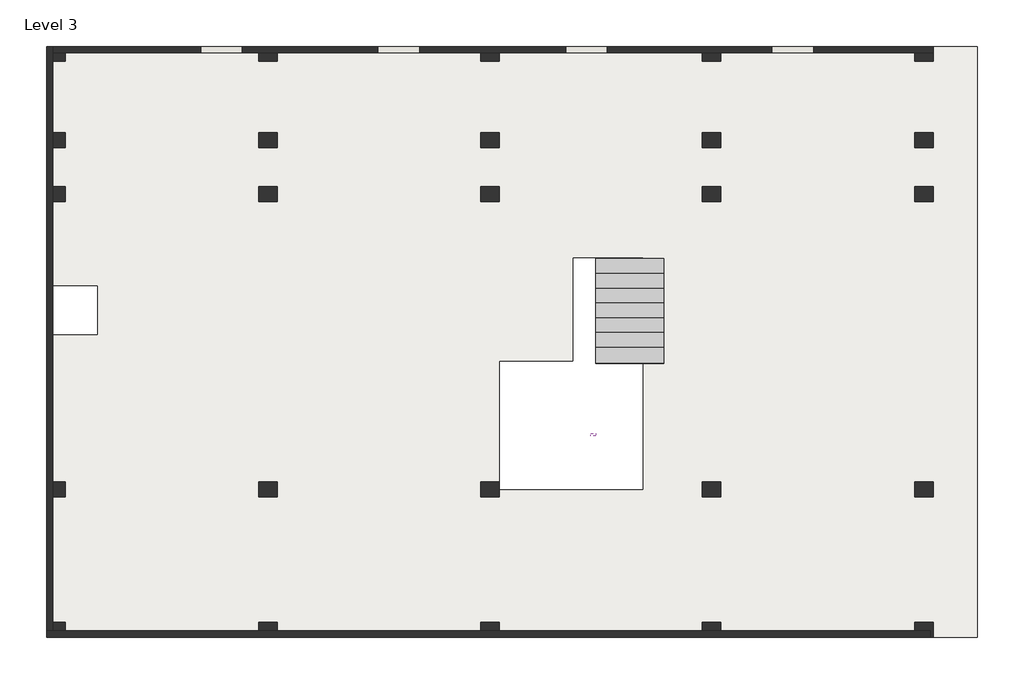
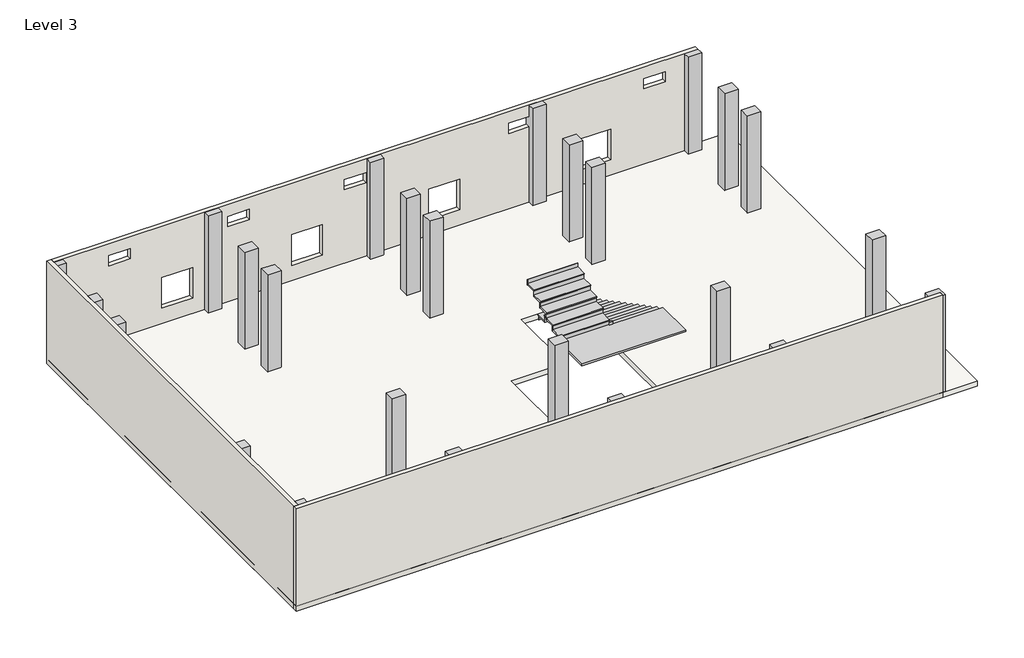
# One storey: 25 columns, 3 walls, 1 member, 1 slab, 1 stair flight.
"""IFC4 building model written with IfcOpenShell, lengths in millimetres."""

from ifc_helpers import new_model, si_unit, frame, origin, place, context, project, spatial, polyline, outline, extrude, faceted_brep, transform, mapped, element, save
from components import column_family_column_family_39b5c8c6, stair_flight_2e5e19c8

model = new_model("IFC4")

# Units and contexts
model_context = context("Model", 3, world=origin())
ifc_project = project(units=[si_unit("LENGTHUNIT", "METRE", prefix="MILLI")], contexts=[model_context])

# Site, building, storey
site = spatial("IfcSite", under=ifc_project)
building = spatial("IfcBuilding", under=site)
storey = spatial("IfcBuildingStorey", under=building, Name="Level 3", Elevation=6096.0)

# Columns
placement = place(None, origin())
element("IfcColumn", 1, ObjectType="column family : column family", at=placement, inside=storey, context=model_context, shape_type="SweptSolid", body=[
    extrude(outline(polyline([(-12064.0425534, 2926.4168492), (-12318.0425534, 2926.4168492), (-12318.0425534, 3104.2168492), (-12064.0425534, 3104.2168492), (-12064.0425534, 2926.4168492)])), frame((0.0, 0.0, 6101.0), z_axis=(0.0, 0.0, 1.0), x_axis=(1.0, 0.0, 0.0)), (0.0, 0.0, 1.0), 3038.0),
])
element("IfcColumn", 2, ObjectType="column family : column family", at=placement, inside=storey, context=model_context, shape_type="SweptSolid", body=[
    extrude(outline(polyline([(-7682.5425534, 2926.4168492), (-8063.5425534, 2926.4168492), (-8063.5425534, 3104.2168492), (-7682.5425534, 3104.2168492), (-7682.5425534, 2926.4168492)])), frame((0.0, 0.0, 6101.0), z_axis=(0.0, 0.0, 1.0), x_axis=(1.0, 0.0, 0.0)), (0.0, 0.0, 1.0), 3038.0),
])
element("IfcColumn", 3, ObjectType="column family : column family", at=placement, inside=storey, context=model_context, shape_type="SweptSolid", body=[
    extrude(outline(polyline([(-3110.5425534, 2926.4168492), (-3491.5425534, 2926.4168492), (-3491.5425534, 3104.2168492), (-3110.5425534, 3104.2168492), (-3110.5425534, 2926.4168492)])), frame((0.0, 0.0, 6101.0), z_axis=(0.0, 0.0, 1.0), x_axis=(1.0, 0.0, 0.0)), (0.0, 0.0, 1.0), 3038.0),
])
element("IfcColumn", 4, ObjectType="column family : column family", at=placement, inside=storey, context=model_context, shape_type="Brep", body=[
    faceted_brep([(1461.4574466, 2926.4168492, 6101.0), (1080.4574466, 2926.4168492, 6101.0), (1080.4574466, 3104.2168492, 6101.0), (1461.4574466, 3104.2168492, 6101.0), (1461.4574466, 2926.4168492, 9139.0), (1461.4574466, 3104.2168492, 9139.0), (1080.4574466, 2926.4168492, 9139.0), (1080.4574466, 3104.2168492, 9139.0), (1080.4574466, 3104.2168492, 8797.4055795), (1080.4574466, 3231.2168492, 8797.4055795), (1080.4574466, 3231.2168492, 8492.6055795), (1080.4574466, 3104.2168492, 8492.6055795), (1118.5574466, 3231.2168492, 8797.4055795), (1118.5574466, 3231.2168492, 8492.6055795), (1118.5574466, 3104.2168492, 8492.6055795), (1118.5574466, 3104.2168492, 8797.4055795)], [[[0, 1, 2, 3]], [[4, 0, 3, 5]], [[1, 0, 4, 6]], [[1, 6, 7, 8, 9, 10, 11, 2]], [[10, 9, 12, 13]], [[6, 4, 5, 7]], [[14, 15, 8, 7, 5, 3, 2, 11]], [[13, 14, 11, 10]], [[15, 14, 13, 12]], [[15, 12, 9, 8]]]),
])
element("IfcColumn", 5, ObjectType="column family : column family", at=placement, inside=storey, context=model_context, shape_type="SweptSolid", body=[
    extrude(outline(polyline([(5842.9574466, 2926.4168492), (5461.9574466, 2926.4168492), (5461.9574466, 3104.2168492), (5842.9574466, 3104.2168492), (5842.9574466, 2926.4168492)])), frame((0.0, 0.0, 6101.0), z_axis=(0.0, 0.0, 1.0), x_axis=(1.0, 0.0, 0.0)), (0.0, 0.0, 1.0), 3038.0),
])
element("IfcColumn", 6, ObjectType="column family : column family", at=placement, inside=storey, context=model_context, shape_type="SweptSolid", body=[
    extrude(outline(polyline([(-12064.0425534, 335.6168492), (-12064.0425534, 30.8168492), (-12318.0425534, 30.8168492), (-12318.0425534, 335.6168492), (-12064.0425534, 335.6168492)])), frame((0.0, 0.0, 6101.0), z_axis=(0.0, 0.0, 1.0), x_axis=(1.0, 0.0, 0.0)), (0.0, 0.0, 1.0), 3038.0),
])
element("IfcColumn", 7, ObjectType="column family : column family", at=placement, inside=storey, context=model_context, shape_type="SweptSolid", body=[
    extrude(outline(polyline([(-12064.0425534, 1449.6754758), (-12064.0425534, 1144.8754758), (-12318.0425534, 1144.8754758), (-12318.0425534, 1449.6754758), (-12064.0425534, 1449.6754758)])), frame((0.0, 0.0, 6101.0), z_axis=(0.0, 0.0, 1.0), x_axis=(1.0, 0.0, 0.0)), (0.0, 0.0, 1.0), 3038.0),
])
element("IfcColumn", 8, ObjectType="column family : column family", at=placement, inside=storey, context=model_context, shape_type="SweptSolid", body=[
    extrude(outline(polyline([(-12064.0425534, -5760.3831508), (-12064.0425534, -6065.1831508), (-12318.0425534, -6065.1831508), (-12318.0425534, -5760.3831508), (-12064.0425534, -5760.3831508)])), frame((0.0, 0.0, 6101.0), z_axis=(0.0, 0.0, 1.0), x_axis=(1.0, 0.0, 0.0)), (0.0, 0.0, 1.0), 3038.0),
])
element("IfcColumn", 9, ObjectType="column family : column family", at=placement, inside=storey, context=model_context, shape_type="SweptSolid", body=[
    extrude(outline(polyline([(-12064.0425534, -8655.9831508), (-12064.0425534, -8833.7831508), (-12318.0425534, -8833.7831508), (-12318.0425534, -8655.9831508), (-12064.0425534, -8655.9831508)])), frame((0.0, 0.0, 6101.0), z_axis=(0.0, 0.0, 1.0), x_axis=(1.0, 0.0, 0.0)), (0.0, 0.0, 1.0), 3038.0),
])
element("IfcColumn", 10, ObjectType="column family : column family", at=placement, inside=storey, context=model_context, shape_type="SweptSolid", body=[
    extrude(outline(polyline([(5842.9574466, 335.6168492), (5842.9574466, 30.8168492), (5461.9574466, 30.8168492), (5461.9574466, 335.6168492), (5842.9574466, 335.6168492)])), frame((0.0, 0.0, 6101.0), z_axis=(0.0, 0.0, 1.0), x_axis=(1.0, 0.0, 0.0)), (0.0, 0.0, 1.0), 3038.0),
])
element("IfcColumn", 11, ObjectType="column family : column family", at=placement, inside=storey, context=model_context, shape_type="SweptSolid", body=[
    extrude(outline(polyline([(5842.9574466, 1449.6754758), (5842.9574466, 1144.8754758), (5461.9574466, 1144.8754758), (5461.9574466, 1449.6754758), (5842.9574466, 1449.6754758)])), frame((0.0, 0.0, 6101.0), z_axis=(0.0, 0.0, 1.0), x_axis=(1.0, 0.0, 0.0)), (0.0, 0.0, 1.0), 3038.0),
])
element("IfcColumn", 12, ObjectType="column family : column family", at=placement, inside=storey, context=model_context, shape_type="SweptSolid", body=[
    extrude(outline(polyline([(5842.9574466, -5760.3831508), (5842.9574466, -6065.1831508), (5461.9574466, -6065.1831508), (5461.9574466, -5760.3831508), (5842.9574466, -5760.3831508)])), frame((0.0, 0.0, 6101.0), z_axis=(0.0, 0.0, 1.0), x_axis=(1.0, 0.0, 0.0)), (0.0, 0.0, 1.0), 3038.0),
])
element("IfcColumn", 13, ObjectType="column family : column family", at=placement, inside=storey, context=model_context, shape_type="SweptSolid", body=[
    extrude(outline(polyline([(5842.9574466, -8655.9831508), (5842.9574466, -8960.7831508), (5779.4574466, -8960.7831508), (5779.4574466, -8833.7831508), (5461.9574466, -8833.7831508), (5461.9574466, -8655.9831508), (5842.9574466, -8655.9831508)])), frame((0.0, 0.0, 6101.0), z_axis=(0.0, 0.0, 1.0), x_axis=(1.0, 0.0, 0.0)), (0.0, 0.0, 1.0), 3038.0),
])
element("IfcColumn", 14, ObjectType="column family : column family", at=placement, inside=storey, context=model_context, shape_type="SweptSolid", body=[
    extrude(outline(polyline([(-8063.5425534, -8655.9831508), (-7682.5425534, -8655.9831508), (-7682.5425534, -8833.7831508), (-8063.5425534, -8833.7831508), (-8063.5425534, -8655.9831508)])), frame((0.0, 0.0, 6101.0), z_axis=(0.0, 0.0, 1.0), x_axis=(1.0, 0.0, 0.0)), (0.0, 0.0, 1.0), 3038.0),
])
element("IfcColumn", 15, ObjectType="column family : column family", at=placement, inside=storey, context=model_context, shape_type="SweptSolid", body=[
    extrude(outline(polyline([(-3491.5425534, -8655.9831508), (-3110.5425534, -8655.9831508), (-3110.5425534, -8833.7831508), (-3491.5425534, -8833.7831508), (-3491.5425534, -8655.9831508)])), frame((0.0, 0.0, 6101.0), z_axis=(0.0, 0.0, 1.0), x_axis=(1.0, 0.0, 0.0)), (0.0, 0.0, 1.0), 3038.0),
])
element("IfcColumn", 16, ObjectType="column family : column family", at=placement, inside=storey, context=model_context, shape_type="SweptSolid", body=[
    extrude(outline(polyline([(1080.4574466, -8655.9831508), (1461.4574466, -8655.9831508), (1461.4574466, -8833.7831508), (1080.4574466, -8833.7831508), (1080.4574466, -8655.9831508)])), frame((0.0, 0.0, 6101.0), z_axis=(0.0, 0.0, 1.0), x_axis=(1.0, 0.0, 0.0)), (0.0, 0.0, 1.0), 3038.0),
])
column_family_column_family_shape = column_family_column_family_39b5c8c6(model_context)
element("IfcColumn", 17, ObjectType="column family : column family", at=placement, inside=storey, context=model_context, shape_type="MappedRepresentation", body=[
    mapped(column_family_column_family_shape, transform((-7928.6704001, 183.2168492, 0.0), x_axis=(1.0, 0.0, 0.0), y_axis=(0.0, 1.0, 0.0), z_axis=(0.0, 0.0, 1.0))),
])
element("IfcColumn", 18, ObjectType="column family : column family", at=placement, inside=storey, context=model_context, shape_type="MappedRepresentation", body=[
    mapped(column_family_column_family_shape, transform((-3356.6704001, 183.2168492, 0.0), x_axis=(1.0, 0.0, 0.0), y_axis=(0.0, 1.0, 0.0), z_axis=(0.0, 0.0, 1.0))),
])
element("IfcColumn", 19, ObjectType="column family : column family", at=placement, inside=storey, context=model_context, shape_type="MappedRepresentation", body=[
    mapped(column_family_column_family_shape, transform((1215.3295999, 183.2168492, 0.0), x_axis=(1.0, 0.0, 0.0), y_axis=(0.0, 1.0, 0.0), z_axis=(0.0, 0.0, 1.0))),
])
element("IfcColumn", 20, ObjectType="column family : column family", at=placement, inside=storey, context=model_context, shape_type="MappedRepresentation", body=[
    mapped(column_family_column_family_shape, transform((1215.3295999, 1297.2754758, 0.0), x_axis=(1.0, 0.0, 0.0), y_axis=(0.0, 1.0, 0.0), z_axis=(0.0, 0.0, 1.0))),
])
element("IfcColumn", 21, ObjectType="column family : column family", at=placement, inside=storey, context=model_context, shape_type="MappedRepresentation", body=[
    mapped(column_family_column_family_shape, transform((-3356.6704001, 1297.2754758, 0.0), x_axis=(1.0, 0.0, 0.0), y_axis=(0.0, 1.0, 0.0), z_axis=(0.0, 0.0, 1.0))),
])
element("IfcColumn", 22, ObjectType="column family : column family", at=placement, inside=storey, context=model_context, shape_type="MappedRepresentation", body=[
    mapped(column_family_column_family_shape, transform((-7928.6704001, 1297.2754758, 0.0), x_axis=(1.0, 0.0, 0.0), y_axis=(0.0, 1.0, 0.0), z_axis=(0.0, 0.0, 1.0))),
])
element("IfcColumn", 23, ObjectType="column family : column family", at=placement, inside=storey, context=model_context, shape_type="MappedRepresentation", body=[
    mapped(column_family_column_family_shape, transform((-7928.6704001, -5912.7831508, 0.0), x_axis=(1.0, 0.0, 0.0), y_axis=(0.0, 1.0, 0.0), z_axis=(0.0, 0.0, 1.0))),
])
element("IfcColumn", 24, ObjectType="column family : column family", at=placement, inside=storey, context=model_context, shape_type="MappedRepresentation", body=[
    mapped(column_family_column_family_shape, transform((-3356.6704001, -5912.7831508, 0.0), x_axis=(1.0, 0.0, 0.0), y_axis=(0.0, 1.0, 0.0), z_axis=(0.0, 0.0, 1.0))),
])
element("IfcColumn", 25, ObjectType="column family : column family", at=placement, inside=storey, context=model_context, shape_type="MappedRepresentation", body=[
    mapped(column_family_column_family_shape, transform((1215.3295999, -5912.7831508, 0.0), x_axis=(1.0, 0.0, 0.0), y_axis=(0.0, 1.0, 0.0), z_axis=(0.0, 0.0, 1.0))),
])

# Member
element("IfcMember", 26, ObjectType="Stringer - 2\" Width", at=placement, inside=storey, context=model_context, shape_type="SweptSolid", body=[
    extrude(outline(polyline([(-1121.360394, -4757.0831508), (-1121.360394, -4807.8831508), (-1222.960394, -4807.8831508), (-1222.960394, -4757.0831508), (-1121.360394, -4757.0831508)])), frame((0.0, 0.0, 7952.8736842), z_axis=(0.0, 0.0, 1.0), x_axis=(1.0, 0.0, 0.0)), (0.0, 0.0, 1.0), 304.8),
])

# Slab
element("IfcSlab", 27, ObjectType="Generic - 12\"", at=placement, inside=storey, context=model_context, shape_type="SweptSolid", body=[
    extrude(outline(polyline([(6757.3574466, 3231.2168492), (6757.3574466, -8960.7831508), (-12445.0425534, -8960.7831508), (-12445.0425534, 3231.2168492), (6757.3574466, 3231.2168492)]), holes=[polyline([(-3096.210394, -5912.7831508), (-144.730394, -5912.7831508), (-144.730394, -1135.0431508), (-1578.560394, -1135.0431508), (-1578.560394, -3273.1068434), (-3096.210394, -3273.1068434), (-3096.210394, -5912.7831508)]), polyline([(-11403.6425534, -1709.0831508), (-12318.0425534, -1709.0831508), (-12318.0425534, -2712.3831508), (-11403.6425534, -2712.3831508), (-11403.6425534, -1709.0831508)])]), frame((0.0, 0.0, 6096.0), z_axis=(0.0, 0.0, 1.0), x_axis=(1.0, 0.0, 0.0)), (0.0, 0.0, 1.0), 152.4),
])

# Stair flight
stair_flight_shape = stair_flight_2e5e19c8(model_context)
element("IfcStairFlight", 28, ObjectType="2\" Tread 1\" Nosing 1/4\" Riser", at=placement, inside=storey, context=model_context, shape_type="MappedRepresentation", body=[
    mapped(stair_flight_shape, transform((0.0, 0.0, 0.0), x_axis=(1.0, 0.0, 0.0), y_axis=(0.0, 1.0, 0.0), z_axis=(0.0, 0.0, 1.0))),
])

# Walls
element("IfcWall", 29, ObjectType="Generic - 5\"", at=placement, inside=storey, context=model_context, shape_type="Brep", body=[
    faceted_brep([(-12445.0425534, -8960.7831508, 6096.0), (5779.4574466, -8960.7831508, 6096.0), (5779.4574466, -8960.7831508, 6101.0), (5779.4574466, -8960.7831508, 9139.0), (5779.4574466, -8960.7831508, 9144.0), (-12445.0425534, -8960.7831508, 9144.0), (-12445.0425534, -8833.7831508, 6096.0), (-12445.0425534, -8833.7831508, 9144.0), (-12318.0425534, -8833.7831508, 9144.0), (5779.4574466, -8833.7831508, 9144.0), (5779.4574466, -8833.7831508, 9139.0), (5779.4574466, -8833.7831508, 6101.0), (5779.4574466, -8833.7831508, 6096.0), (-12318.0425534, -8833.7831508, 6096.0)], [[[0, 1, 2, 3, 4, 5]], [[6, 7, 8, 9, 10, 11, 12, 13]], [[1, 0, 6, 13, 12]], [[4, 3, 2, 1, 12, 11, 10, 9]], [[5, 4, 9, 8, 7]], [[0, 5, 7, 6]]]),
])
element("IfcWall", 30, ObjectType="Generic - 5\"", at=placement, inside=storey, context=model_context, shape_type="Brep", body=[
    faceted_brep([(-12318.0425534, -8833.7831508, 6096.0), (-12318.0425534, 3104.2168492, 6096.0), (-12318.0425534, 3231.2168492, 6096.0), (-12318.0425534, 3231.2168492, 9144.0), (-12318.0425534, 3104.2168492, 9144.0), (-12318.0425534, -8833.7831508, 9144.0), (-12318.0425534, -8833.7831508, 9139.0), (-12318.0425534, -8833.7831508, 6101.0), (-12445.0425534, -8833.7831508, 6096.0), (-12445.0425534, -8833.7831508, 9144.0), (-12445.0425534, 3231.2168492, 9144.0), (-12445.0425534, 3231.2168492, 6096.0)], [[[0, 1, 2, 3, 4, 5, 6, 7]], [[8, 9, 10, 11]], [[2, 1, 0, 8, 11]], [[5, 4, 3, 10, 9]], [[0, 7, 6, 5, 9, 8]], [[3, 2, 11, 10]]]),
])
element("IfcWall", 31, ObjectType="Generic - 5\"", at=placement, inside=storey, context=model_context, shape_type="Brep", body=[
    faceted_brep([(-12318.0425534, 3104.2168492, 6096.0), (5842.9574466, 3104.2168492, 6096.0), (5842.9574466, 3104.2168492, 6101.0), (5842.9574466, 3104.2168492, 9139.0), (5842.9574466, 3104.2168492, 9144.0), (-12318.0425534, 3104.2168492, 9144.0), (-12318.0425534, 3104.2168492, 9139.0), (-12318.0425534, 3104.2168492, 6101.0), (4318.9574466, 3104.2168492, 8797.4055795), (4928.5574466, 3104.2168492, 8797.4055795), (4928.5574466, 3104.2168492, 8492.6055795), (4318.9574466, 3104.2168492, 8492.6055795), (508.9574466, 3104.2168492, 8797.4055795), (1080.4574466, 3104.2168492, 8797.4055795), (1118.5574466, 3104.2168492, 8797.4055795), (1118.5574466, 3104.2168492, 8492.6055795), (1080.4574466, 3104.2168492, 8492.6055795), (508.9574466, 3104.2168492, 8492.6055795), (-4120.1925534, 3104.2168492, 8740.2555795), (-3510.5925534, 3104.2168492, 8740.2555795), (-3510.5925534, 3104.2168492, 8435.4555795), (-4120.1925534, 3104.2168492, 8435.4555795), (3379.1574466, 3104.2168492, 7618.9023039), (3379.1574466, 3104.2168492, 6704.5023039), (2515.5574466, 3104.2168492, 6704.5023039), (2515.5574466, 3104.2168492, 7618.9023039), (-874.980394, 3104.2168492, 7618.9023039), (-874.980394, 3104.2168492, 6704.5023039), (-1738.580394, 3104.2168492, 6704.5023039), (-1738.580394, 3104.2168492, 7618.9023039), (-7415.8425534, 3104.2168492, 8797.4055795), (-6806.2425534, 3104.2168492, 8797.4055795), (-6806.2425534, 3104.2168492, 8492.6055795), (-7415.8425534, 3104.2168492, 8492.6055795), (-10768.6425534, 3104.2168492, 8797.4055795), (-10159.0425534, 3104.2168492, 8797.4055795), (-10159.0425534, 3104.2168492, 8492.6055795), (-10768.6425534, 3104.2168492, 8492.6055795), (-4745.6675534, 3104.2168492, 7618.9023039), (-4745.6675534, 3104.2168492, 6704.5023039), (-5609.2675534, 3104.2168492, 6704.5023039), (-5609.2675534, 3104.2168492, 7618.9023039), (-8403.2675534, 3104.2168492, 7618.9023039), (-8403.2675534, 3104.2168492, 6704.5023039), (-9266.8675534, 3104.2168492, 6704.5023039), (-9266.8675534, 3104.2168492, 7618.9023039), (-12318.0425534, 3231.2168492, 6096.0), (-12318.0425534, 3231.2168492, 9144.0), (5842.9574466, 3231.2168492, 9144.0), (5842.9574466, 3231.2168492, 6096.0), (4318.9574466, 3231.2168492, 8797.4055795), (4318.9574466, 3231.2168492, 8492.6055795), (4928.5574466, 3231.2168492, 8492.6055795), (4928.5574466, 3231.2168492, 8797.4055795), (508.9574466, 3231.2168492, 8797.4055795), (508.9574466, 3231.2168492, 8492.6055795), (1080.4574466, 3231.2168492, 8492.6055795), (1118.5574466, 3231.2168492, 8492.6055795), (1118.5574466, 3231.2168492, 8797.4055795), (1080.4574466, 3231.2168492, 8797.4055795), (-4120.1925534, 3231.2168492, 8740.2555795), (-4120.1925534, 3231.2168492, 8435.4555795), (-3510.5925534, 3231.2168492, 8435.4555795), (-3510.5925534, 3231.2168492, 8740.2555795), (3379.1574466, 3231.2168492, 7618.9023039), (2515.5574466, 3231.2168492, 7618.9023039), (2515.5574466, 3231.2168492, 6704.5023039), (3379.1574466, 3231.2168492, 6704.5023039), (-874.980394, 3231.2168492, 7618.9023039), (-1738.580394, 3231.2168492, 7618.9023039), (-1738.580394, 3231.2168492, 6704.5023039), (-874.980394, 3231.2168492, 6704.5023039), (-7415.8425534, 3231.2168492, 8797.4055795), (-7415.8425534, 3231.2168492, 8492.6055795), (-6806.2425534, 3231.2168492, 8492.6055795), (-6806.2425534, 3231.2168492, 8797.4055795), (-10768.6425534, 3231.2168492, 8797.4055795), (-10768.6425534, 3231.2168492, 8492.6055795), (-10159.0425534, 3231.2168492, 8492.6055795), (-10159.0425534, 3231.2168492, 8797.4055795), (-4745.6675534, 3231.2168492, 7618.9023039), (-5609.2675534, 3231.2168492, 7618.9023039), (-5609.2675534, 3231.2168492, 6704.5023039), (-4745.6675534, 3231.2168492, 6704.5023039), (-8403.2675534, 3231.2168492, 7618.9023039), (-9266.8675534, 3231.2168492, 7618.9023039), (-9266.8675534, 3231.2168492, 6704.5023039), (-8403.2675534, 3231.2168492, 6704.5023039)], [[[0, 1, 2, 3, 4, 5, 6, 7], [8, 9, 10, 11], [12, 13, 14, 15, 16, 17], [18, 19, 20, 21], [22, 23, 24, 25], [26, 27, 28, 29], [30, 31, 32, 33], [34, 35, 36, 37], [38, 39, 40, 41], [42, 43, 44, 45]], [[46, 47, 48, 49], [50, 51, 52, 53], [54, 55, 56, 57, 58, 59], [60, 61, 62, 63], [64, 65, 66, 67], [68, 69, 70, 71], [72, 73, 74, 75], [76, 77, 78, 79], [80, 81, 82, 83], [84, 85, 86, 87]], [[1, 0, 46, 49]], [[4, 3, 2, 1, 49, 48]], [[5, 4, 48, 47]], [[0, 7, 6, 5, 47, 46]], [[51, 50, 8, 11]], [[52, 51, 11, 10]], [[53, 52, 10, 9]], [[50, 53, 9, 8]], [[55, 54, 12, 17]], [[57, 56, 55, 17, 16, 15]], [[58, 57, 15, 14]], [[54, 59, 58, 14, 13, 12]], [[61, 60, 18, 21]], [[62, 61, 21, 20]], [[63, 62, 20, 19]], [[60, 63, 19, 18]], [[23, 22, 64, 67]], [[24, 23, 67, 66]], [[25, 24, 66, 65]], [[22, 25, 65, 64]], [[27, 26, 68, 71]], [[28, 27, 71, 70]], [[29, 28, 70, 69]], [[26, 29, 69, 68]], [[73, 72, 30, 33]], [[74, 73, 33, 32]], [[75, 74, 32, 31]], [[72, 75, 31, 30]], [[77, 76, 34, 37]], [[78, 77, 37, 36]], [[79, 78, 36, 35]], [[76, 79, 35, 34]], [[39, 38, 80, 83]], [[40, 39, 83, 82]], [[41, 40, 82, 81]], [[38, 41, 81, 80]], [[43, 42, 84, 87]], [[44, 43, 87, 86]], [[45, 44, 86, 85]], [[42, 45, 85, 84]]]),
])

save(model, "model.ifc")

# Revit data of these elements
# Type "column family : column family"
#   w2 [instance default] = 0' - 9.88189"
#   w1 [instance default] = 0' - 9.01575"
#   Depth = 1' - 11.62205"
#   Width = 1' - 11.62205"
# Type "Generic - 12\""
#   Assembly Code = "B1010"
#   Function = 0
#   Layers, outside or top first: 0' - 6" no material (function 1)
# Type "Generic - 5\""
#   Assembly Code = "B2010"
#   Layers, outside or top first: 0' - 5" no material (function 1)
# Elements 1, 2, 3, 4, 5, 6, 7, 8, 9, 14, 15, 16 (IfcColumn, "column family : column family")
#   w2 = 1' - 0"
#   w1 = 1' - 3"
#   Phase Created = New Construction
#   Materials on its faces: "Default Wall"
# Elements 10, 11, 12, 17, 18, 19, 20, 21, 22, 23, 24, 25 (IfcColumn, "column family : column family")
#   w2 = 1' - 0"
#   w1 = 1' - 3"
#   Phase Created = New Construction
# Element 13 (IfcColumn, "column family : column family")
#   w2 = 1' - 0"
#   w1 = 1' - 3"
#   Phase Created = New Construction
#   Materials on its faces: "Default Wall", "cream colour"
# Element 26 (IfcMember, "Stringer - 2\" Width")
#   Phase Created = New Construction
# Element 27 (IfcSlab, "Generic - 12\"")
#   Height Offset From Level = 0' - 6"
#   Phase Created = New Construction
#   Materials on its faces: "Default Floor", "cream colour", "Wood - Stained"
# Element 28 (IfcStairFlight, "2\" Tread 1\" Nosing 1/4\" Riser")
#   Phase Created = New Construction
# Elements 29, 30, 31 (IfcWall, "Generic - 5\"")
#   Top Offset = 0' - 0"
#   Base Offset = 0' - 0"
#   wall height = 10' - 0"
#   Phase Created = New Construction
#   Base Constraint = Level 3
#   Top Constraint = Level 4
#   Materials on its faces: "Default Wall", "cream colour"
# Materials
#   "Default Wall": colour RGB 128 128 128, transparency 0, Cost = 0
#   "cream colour": class "Generic", colour RGB 255 166 166, transparency 0, Cost = 0
#   "Default Floor": colour RGB 128 128 128, transparency 0, Cost = 0
#   "Wood - Stained": class "Wood", colour RGB 224 178 126, transparency 0, Cost = 0
